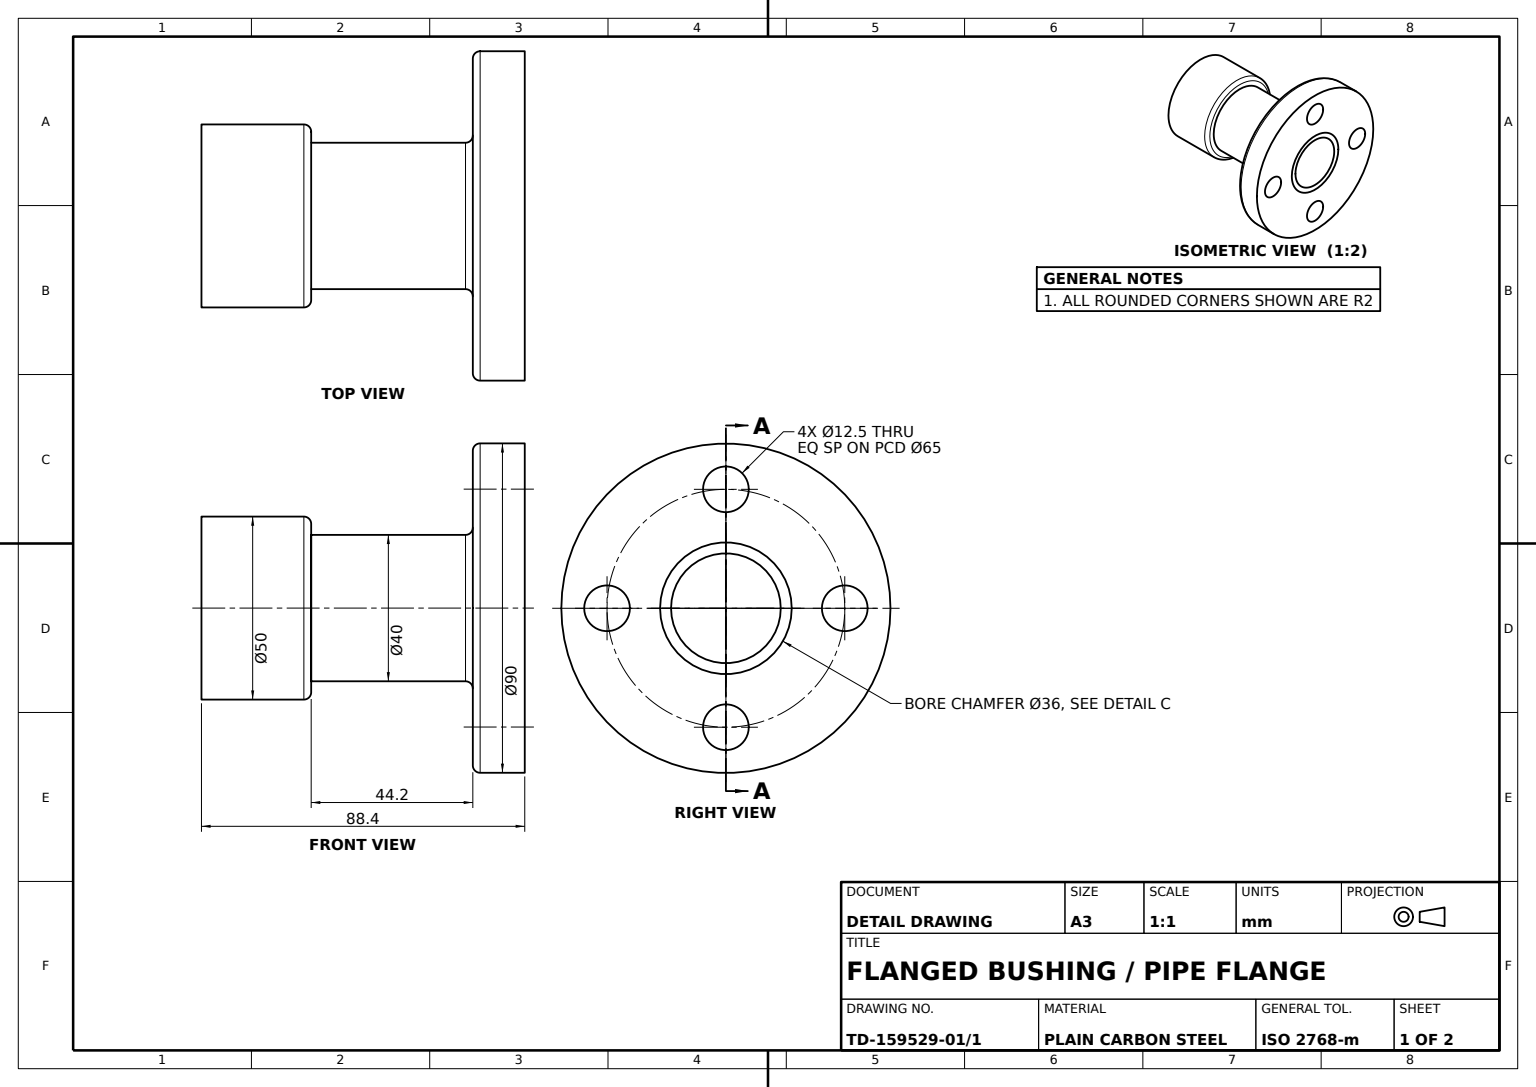
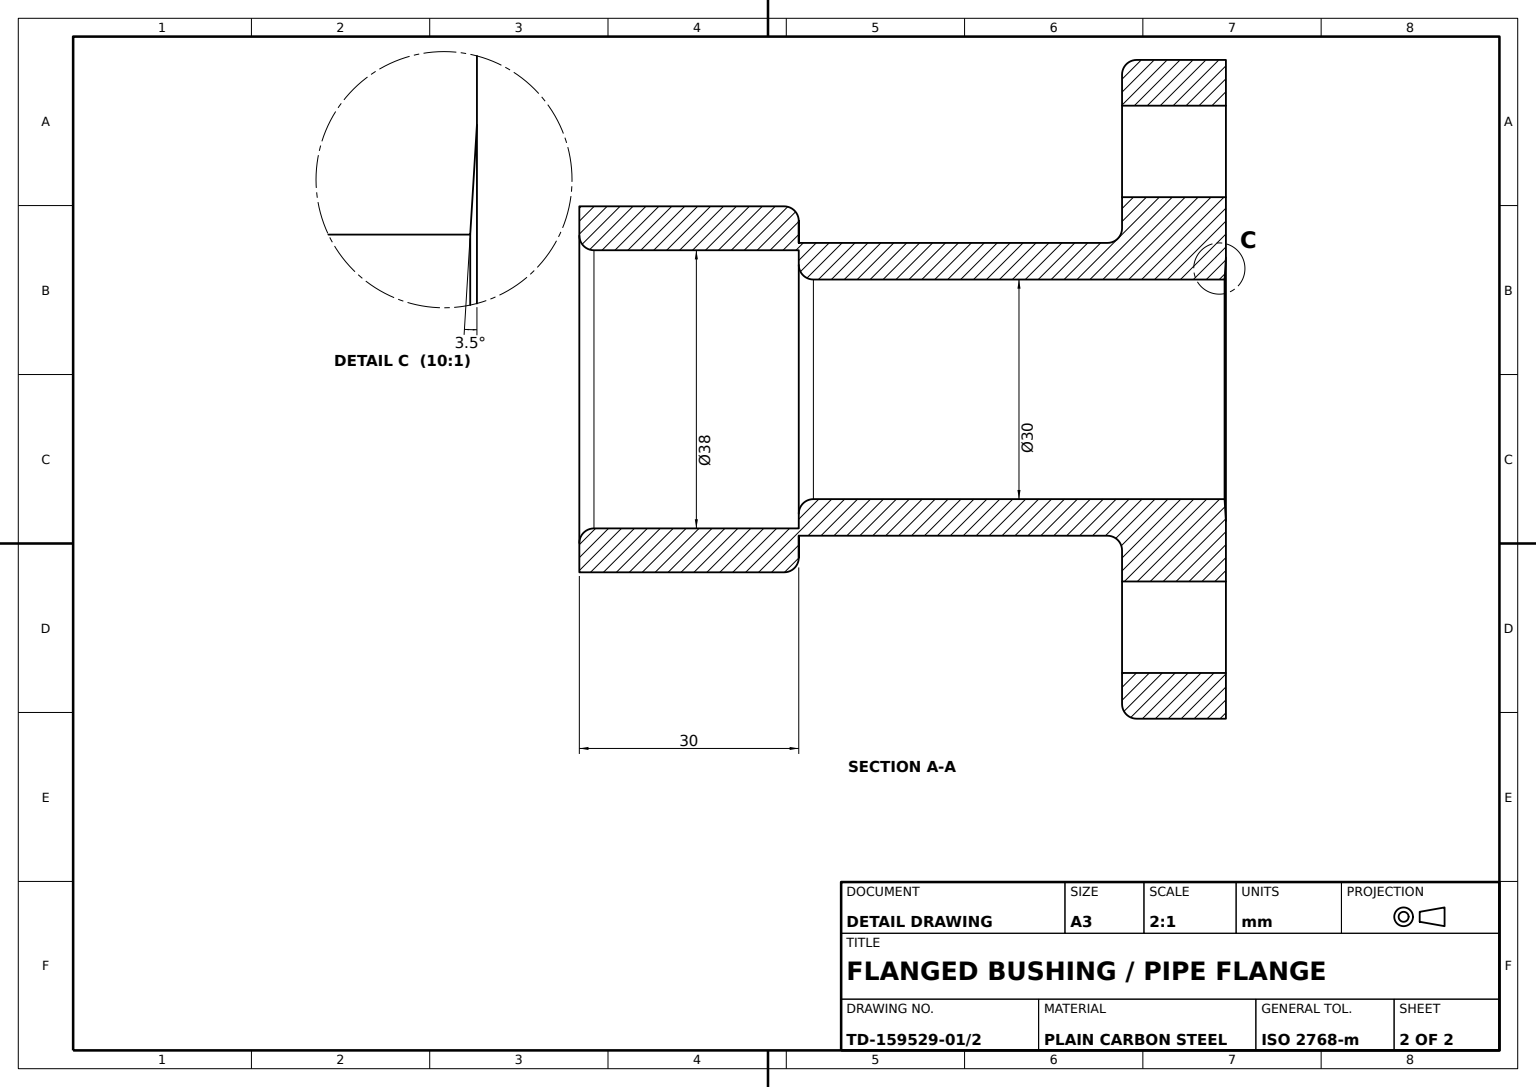
from build123d import *

# Parameters (mm, degrees)
FLANGE_PROFILE_90_R        = 45
FLANGE_90_DEPTH            = 14.2
FLANGE_HOLES_SKETCH_R      = 6.25
FLANGE_HOLES_4X_12_5_DEPTH = 14.2
SHANK_PROFILE_40_R         = 20
SHANK_40_DEPTH             = 44.2
BORE_PROFILE_30_R          = 15
THROUGH_BORE_30_DEPTH      = 87.374533284
BORE_CHAMFER_3MM_SIZE      = 3
BORE_CHAMFER_3MM_SIZE2     = 0.18348786
COLLAR_PROFILE_50_38_R     = 25
COLLAR_PROFILE_50_38_R_2   = 19
END_COLLAR_50_DEPTH        = 30
FLANGE_EDGE_FILLET_R2_R    = 2
FLANGE_SHANK_FILLET_R2_R   = 2
COLLAR_FILLET_R2_A_R       = 2
SHANK_BORE_FILLET_R2_R     = 2
COLLAR_FILLET_R2_B_R       = 2


with BuildPart() as part:
    # Flange Profile Ø90 → Flange Ø90 (new body)
    with BuildSketch(Plane.XY):
        Circle(FLANGE_PROFILE_90_R)
    extrude(amount=FLANGE_90_DEPTH)

    # Flange Holes Sketch → Flange Holes 4xØ12.5 (cut)
    with BuildSketch(Plane.XY.offset(14.2)):
        with Locations((0, 32.5)):
            Circle(FLANGE_HOLES_SKETCH_R)
        with Locations((0, -32.5)):
            Circle(FLANGE_HOLES_SKETCH_R)
        with Locations((-32.5, 0)):
            Circle(FLANGE_HOLES_SKETCH_R)
        with Locations((32.5, 0)):
            Circle(FLANGE_HOLES_SKETCH_R)
    extrude(amount=-FLANGE_HOLES_4X_12_5_DEPTH, mode=Mode.SUBTRACT)

    # Shank Profile Ø40 → Shank Ø40 (add)
    with BuildSketch(Plane.XY.offset(14.2)):
        Circle(SHANK_PROFILE_40_R)
    extrude(amount=SHANK_40_DEPTH)

    # Bore Profile Ø30 → Through Bore Ø30 (cut, through all)
    with BuildSketch(Plane(origin=(0, 0, 0), x_dir=(-1, 0, 0), z_dir=(0, 0, -1))):
        Circle(BORE_PROFILE_30_R)
    extrude(amount=-THROUGH_BORE_30_DEPTH, mode=Mode.SUBTRACT)

    # Bore Chamfer 3mm
    bore_chamfer_3mm_edges = [part.edges().sort_by_distance(p)[0] for p in [
        (15, 0, 0),
    ]]
    bore_chamfer_3mm_side = [part.faces().sort_by_distance(p)[0] for p in [
        (-43.727207794, 0, 0),
    ]]
    chamfer(bore_chamfer_3mm_edges, length=BORE_CHAMFER_3MM_SIZE, length2=BORE_CHAMFER_3MM_SIZE2, reference=bore_chamfer_3mm_side[0])

    # Collar Profile Ø50-Ø38 → End Collar Ø50 (add)
    with BuildSketch(Plane.XY.offset(58.4)):
        Circle(COLLAR_PROFILE_50_38_R)
        Circle(COLLAR_PROFILE_50_38_R_2, mode=Mode.SUBTRACT)
    extrude(amount=END_COLLAR_50_DEPTH)

    # Flange Edge Fillet R2
    flange_edge_fillet_r2_edges = [part.edges().sort_by_distance(p)[0] for p in [
        (-45, 0, 14.2),
    ]]
    fillet(flange_edge_fillet_r2_edges, radius=FLANGE_EDGE_FILLET_R2_R)

    # Flange-Shank Fillet R2
    flange_shank_fillet_r2_edges = [part.edges().sort_by_distance(p)[0] for p in [
        (-20, 0, 14.2),
    ]]
    fillet(flange_shank_fillet_r2_edges, radius=FLANGE_SHANK_FILLET_R2_R)

    # Collar Fillet R2 A
    collar_fillet_r2_a_edges = [part.edges().sort_by_distance(p)[0] for p in [
        (-19, 0, 88.4),
    ]]
    fillet(collar_fillet_r2_a_edges, radius=COLLAR_FILLET_R2_A_R)

    # Shank Bore Fillet R2
    shank_bore_fillet_r2_edges = [part.edges().sort_by_distance(p)[0] for p in [
        (15, 0, 58.4),
    ]]
    fillet(shank_bore_fillet_r2_edges, radius=SHANK_BORE_FILLET_R2_R)

    # Collar Fillet R2 B
    collar_fillet_r2_b_edges = [part.edges().sort_by_distance(p)[0] for p in [
        (-25, 0, 58.4),
    ]]
    fillet(collar_fillet_r2_b_edges, radius=COLLAR_FILLET_R2_B_R)


solid = part.part
